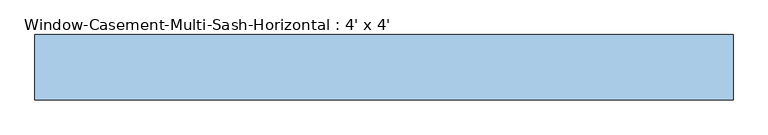
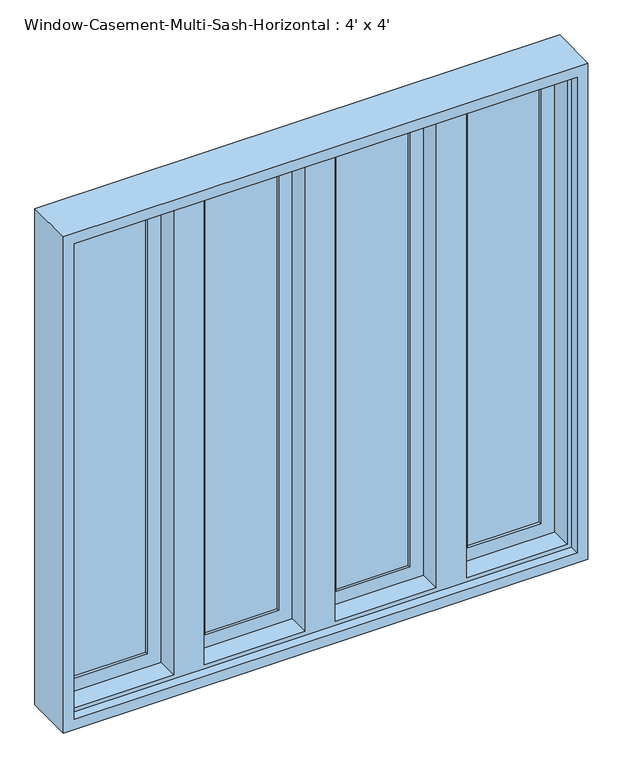
"""IFC4 building model written with IfcOpenShell, lengths in millimetres: window geometry, Window-Casement-Multi-Sash-Horizontal : 4' x 4'."""

from ifc_helpers import new_model, si_unit, frame, origin, place, context, project, spatial, polyline, outline, extrude, faceted_brep, source, transform, mapped, element, save


def window_casement_multi_sash_horizontal_4_x_4_e1d7f736(model_context):
    return source(origin(), model_context, "Body", "SolidModel", [
        extrude(outline(polyline([(2108.2, 330.2), (939.8, 330.2), (939.8, 584.2), (2108.2, 584.2), (2108.2, 330.2)]), holes=[polyline([(2066.3296875, 542.3296875), (981.6703125, 542.3296875), (981.6703125, 372.0703125), (2066.3296875, 372.0703125), (2066.3296875, 542.3296875)])]), frame((0.0, 15.875, 0.0), z_axis=(0.0, 1.0, 0.0), x_axis=(0.0, 0.0, 1.0)), (0.0, 0.0, 1.0), 31.75),
        extrude(outline(polyline([(2108.2, -584.2), (939.8, -584.2), (939.8, -330.2), (2108.2, -330.2), (2108.2, -584.2)]), holes=[polyline([(2066.3296875, -372.0703125), (981.6703125, -372.0703125), (981.6703125, -542.3296875), (2066.3296875, -542.3296875), (2066.3296875, -372.0703125)])]), frame((0.0, 15.875, 0.0), z_axis=(0.0, 1.0, 0.0), x_axis=(0.0, 0.0, 1.0)), (0.0, 0.0, 1.0), 31.75),
        extrude(outline(polyline([(-372.0703125, 41.275), (-372.0703125, 34.925), (-542.3296875, 34.925), (-542.3296875, 41.275), (-372.0703125, 41.275)])), frame((0.0, 0.0, 981.6703125), z_axis=(0.0, 0.0, 1.0), x_axis=(1.0, 0.0, 0.0)), (0.0, 0.0, 1.0), 1084.659375),
        extrude(outline(polyline([(-372.0703125, 28.575), (-372.0703125, 22.225), (-542.3296875, 22.225), (-542.3296875, 28.575), (-372.0703125, 28.575)])), frame((0.0, 0.0, 981.6703125), z_axis=(0.0, 0.0, 1.0), x_axis=(1.0, 0.0, 0.0)), (0.0, 0.0, 1.0), 1084.659375),
        extrude(outline(polyline([(542.3296875, 41.275), (542.3296875, 34.925), (372.0703125, 34.925), (372.0703125, 41.275), (542.3296875, 41.275)])), frame((0.0, 0.0, 981.6703125), z_axis=(0.0, 0.0, 1.0), x_axis=(1.0, 0.0, 0.0)), (0.0, 0.0, 1.0), 1084.659375),
        extrude(outline(polyline([(542.3296875, 28.575), (542.3296875, 22.225), (372.0703125, 22.225), (372.0703125, 28.575), (542.3296875, 28.575)])), frame((0.0, 0.0, 981.6703125), z_axis=(0.0, 0.0, 1.0), x_axis=(1.0, 0.0, 0.0)), (0.0, 0.0, 1.0), 1084.659375),
        extrude(outline(polyline([(-67.2703125, 41.275), (-67.2703125, 34.925), (-237.5296875, 34.925), (-237.5296875, 41.275), (-67.2703125, 41.275)])), frame((0.0, 0.0, 981.6703125), z_axis=(0.0, 0.0, 1.0), x_axis=(1.0, 0.0, 0.0)), (0.0, 0.0, 1.0), 1084.659375),
        extrude(outline(polyline([(-67.2703125, 28.575), (-67.2703125, 22.225), (-237.5296875, 22.225), (-237.5296875, 28.575), (-67.2703125, 28.575)])), frame((0.0, 0.0, 981.6703125), z_axis=(0.0, 0.0, 1.0), x_axis=(1.0, 0.0, 0.0)), (0.0, 0.0, 1.0), 1084.659375),
        extrude(outline(polyline([(237.5296875, 41.275), (237.5296875, 34.925), (67.2703125, 34.925), (67.2703125, 41.275), (237.5296875, 41.275)])), frame((0.0, 0.0, 981.6703125), z_axis=(0.0, 0.0, 1.0), x_axis=(1.0, 0.0, 0.0)), (0.0, 0.0, 1.0), 1084.659375),
        extrude(outline(polyline([(237.5296875, 28.575), (237.5296875, 22.225), (67.2703125, 22.225), (67.2703125, 28.575), (237.5296875, 28.575)])), frame((0.0, 0.0, 981.6703125), z_axis=(0.0, 0.0, 1.0), x_axis=(1.0, 0.0, 0.0)), (0.0, 0.0, 1.0), 1084.659375),
        faceted_brep([(-330.2, 15.875, 2108.2), (-584.2, 15.875, 2108.2), (-584.2, 57.15, 2108.2), (584.2, 57.15, 2108.2), (584.2, 15.875, 2108.2), (330.2, 15.875, 2108.2), (330.2, 53.975, 2108.2), (279.4, 53.975, 2108.2), (279.4, 15.875, 2108.2), (25.4, 15.875, 2108.2), (25.4, 53.975, 2108.2), (-25.4, 53.975, 2108.2), (-25.4, 15.875, 2108.2), (-279.4, 15.875, 2108.2), (-279.4, 53.975, 2108.2), (-330.2, 53.975, 2108.2), (-574.0796875, -34.925, 2098.0796875), (-574.0796875, 15.875, 2098.0796875), (-340.3203125, 15.875, 2098.0796875), (-340.3203125, -34.925, 2098.0796875), (574.0796875, 15.875, 2098.0796875), (574.0796875, -34.925, 2098.0796875), (340.3203125, -34.925, 2098.0796875), (340.3203125, 15.875, 2098.0796875), (-269.2796875, 15.875, 2098.0796875), (-35.5203125, 15.875, 2098.0796875), (-35.5203125, -34.925, 2098.0796875), (-269.2796875, -34.925, 2098.0796875), (35.5203125, 15.875, 2098.0796875), (269.2796875, 15.875, 2098.0796875), (269.2796875, -34.925, 2098.0796875), (35.5203125, -34.925, 2098.0796875), (-584.2, -57.15, 2108.2), (-584.2, -34.925, 2108.2), (584.2, -34.925, 2108.2), (584.2, -57.15, 2108.2), (-609.6, 57.15, 2133.6), (-609.6, -57.15, 2133.6), (609.6, -57.15, 2133.6), (609.6, 57.15, 2133.6), (584.2, 57.15, 939.8), (584.2, 15.875, 939.8), (574.0796875, 15.875, 949.9203125), (574.0796875, -34.925, 949.9203125), (584.2, -34.925, 939.8), (584.2, -57.15, 939.8), (609.6, -57.15, 914.4), (609.6, 57.15, 914.4), (330.2, 15.875, 939.8), (-584.2, 57.15, 939.8), (-584.2, 15.875, 939.8), (-330.2, 15.875, 939.8), (-330.2, 53.975, 939.8), (-279.4, 53.975, 939.8), (-279.4, 15.875, 939.8), (-25.4, 15.875, 939.8), (-25.4, 53.975, 939.8), (25.4, 53.975, 939.8), (25.4, 15.875, 939.8), (279.4, 15.875, 939.8), (279.4, 53.975, 939.8), (330.2, 53.975, 939.8), (340.3203125, 15.875, 949.9203125), (340.3203125, -34.925, 949.9203125), (-574.0796875, 15.875, 949.9203125), (-574.0796875, -34.925, 949.9203125), (-340.3203125, -34.925, 949.9203125), (-340.3203125, 15.875, 949.9203125), (-35.5203125, 15.875, 949.9203125), (-269.2796875, 15.875, 949.9203125), (-269.2796875, -34.925, 949.9203125), (-35.5203125, -34.925, 949.9203125), (269.2796875, 15.875, 949.9203125), (35.5203125, 15.875, 949.9203125), (35.5203125, -34.925, 949.9203125), (269.2796875, -34.925, 949.9203125), (-584.2, -34.925, 939.8), (-584.2, -57.15, 939.8), (-609.6, -57.15, 914.4), (-609.6, 57.15, 914.4)], [[[0, 1, 2, 3, 4, 5, 6, 7, 8, 9, 10, 11, 12, 13, 14, 15]], [[16, 17, 18, 19]], [[20, 21, 22, 23]], [[24, 25, 26, 27]], [[28, 29, 30, 31]], [[32, 33, 34, 35]], [[36, 37, 38, 39]], [[4, 3, 40, 41]], [[21, 20, 42, 43]], [[35, 34, 44, 45]], [[39, 38, 46, 47]], [[48, 41, 40, 49, 50, 51, 52, 53, 54, 55, 56, 57, 58, 59, 60, 61]], [[43, 42, 62, 63]], [[64, 65, 66, 67]], [[68, 69, 70, 71]], [[72, 73, 74, 75]], [[45, 44, 76, 77]], [[47, 46, 78, 79]], [[2, 1, 50, 49]], [[4, 41, 48, 5], [20, 23, 62, 42]], [[50, 1, 0, 51], [64, 67, 18, 17]], [[12, 55, 54, 13], [69, 68, 25, 24]], [[8, 59, 58, 9], [73, 72, 29, 28]], [[17, 16, 65, 64]], [[44, 34, 33, 76], [16, 19, 66, 65], [27, 26, 71, 70], [31, 30, 75, 74], [21, 43, 63, 22]], [[33, 32, 77, 76]], [[38, 37, 78, 46], [32, 35, 45, 77]], [[37, 36, 79, 78]], [[36, 39, 47, 79], [3, 2, 49, 40]], [[18, 67, 66, 19]], [[69, 24, 27, 70]], [[53, 14, 13, 54]], [[14, 53, 52, 15]], [[15, 52, 51, 0]], [[25, 68, 71, 26]], [[73, 28, 31, 74]], [[57, 10, 9, 58]], [[10, 57, 56, 11]], [[11, 56, 55, 12]], [[6, 61, 60, 7]], [[7, 60, 59, 8]], [[29, 72, 75, 30]], [[62, 23, 22, 63]], [[61, 6, 5, 48]]]),
        extrude(outline(polyline([(2108.2, 25.4), (939.8, 25.4), (939.8, 279.4), (2108.2, 279.4), (2108.2, 25.4)]), holes=[polyline([(2066.3296875, 237.5296875), (981.6703125, 237.5296875), (981.6703125, 67.2703125), (2066.3296875, 67.2703125), (2066.3296875, 237.5296875)])]), frame((0.0, 15.875, 0.0), z_axis=(0.0, 1.0, 0.0), x_axis=(0.0, 0.0, 1.0)), (0.0, 0.0, 1.0), 31.75),
        extrude(outline(polyline([(2108.2, -279.4), (939.8, -279.4), (939.8, -25.4), (2108.2, -25.4), (2108.2, -279.4)]), holes=[polyline([(2066.3296875, -67.2703125), (981.6703125, -67.2703125), (981.6703125, -237.5296875), (2066.3296875, -237.5296875), (2066.3296875, -67.2703125)])]), frame((0.0, 15.875, 0.0), z_axis=(0.0, 1.0, 0.0), x_axis=(0.0, 0.0, 1.0)), (0.0, 0.0, 1.0), 31.75),
    ])


if __name__ == "__main__":
    model = new_model("IFC4")
    model_context = context("Model", 3, world=origin())
    ifc_project = project(units=[si_unit("LENGTHUNIT", "METRE", prefix="MILLI")], contexts=[model_context])
    site = spatial("IfcSite", under=ifc_project)
    building = spatial("IfcBuilding", under=site)
    placement = place(None, origin())
    window_casement_multi_sash_horizontal_4_x_4_shape = window_casement_multi_sash_horizontal_4_x_4_e1d7f736(model_context)
    element("IfcWindow", 1, ObjectType="Window-Casement-Multi-Sash-Horizontal : 4' x 4'", at=placement, inside=building, context=model_context, shape_type="MappedRepresentation", body=[
        mapped(window_casement_multi_sash_horizontal_4_x_4_shape, transform((0.0, 0.0, 0.0), x_axis=(1.0, 0.0, 0.0), y_axis=(0.0, 1.0, 0.0), z_axis=(0.0, 0.0, 1.0))),
    ])
    save(model, "model.ifc")

# Revit data of these elements
# Type "Window-Casement-Multi-Sash-Horizontal : 4' x 4'"
#   Type Mark = "W1"
#   Fire Rating = "0.5h"
#   Assembly Code = "B2020100"
#   Analytic Construction = "Double glazing - domestic"
#   Window Inset [instance default] = 0' - 0 5/8"
#   Wall Thickness [instance default] = 0' - 6"
#   Visual Light Transmittance = 0.81
#   Thermal Resistance (R) = 1.8146 (h·ft²·°F)/BTU
#   Solar Heat Gain Coefficient = 0.76
#   Rough Width = 4' - 0 1/2"
#   Rough Height = 4' - 0 1/2"
#   Open Window Width = 1' - 0"
#   Heat Transfer Coefficient (U) = 0.5511 BTU/(h·ft²·°F)
#   Height = 4' - 0"
#   Frame Gap 3 [instance default] = 0' - 1 83/128"
#   Frame Gap 2 [instance default] = 0' - 0 5/8"
#   Frame Gap 1 = 0' - 1 51/128"
#   Default Sill Height = 3' - 0"
#   Width = 4' - 0"
#   Frame Material = Metal - Aluminum
#   Glass Panel Material = Glass
#   Wall Closure = (empty or 0)
# Element 1 (IfcWindow, "Window-Casement-Multi-Sash-Horizontal : 4' x 4'")
#   Wall Thickness = 0' - 4 1/2"
#   Materials on its faces: "Metal - Aluminum", "Glass"
# Materials
#   "Metal - Aluminum": class "Metal", colour RGB 247 247 247, transparency 0
#   "Glass": class "Glass", colour RGB 0 128 192, transparency 0.75, Description = "Soda Lime Glass", Cost = 0
